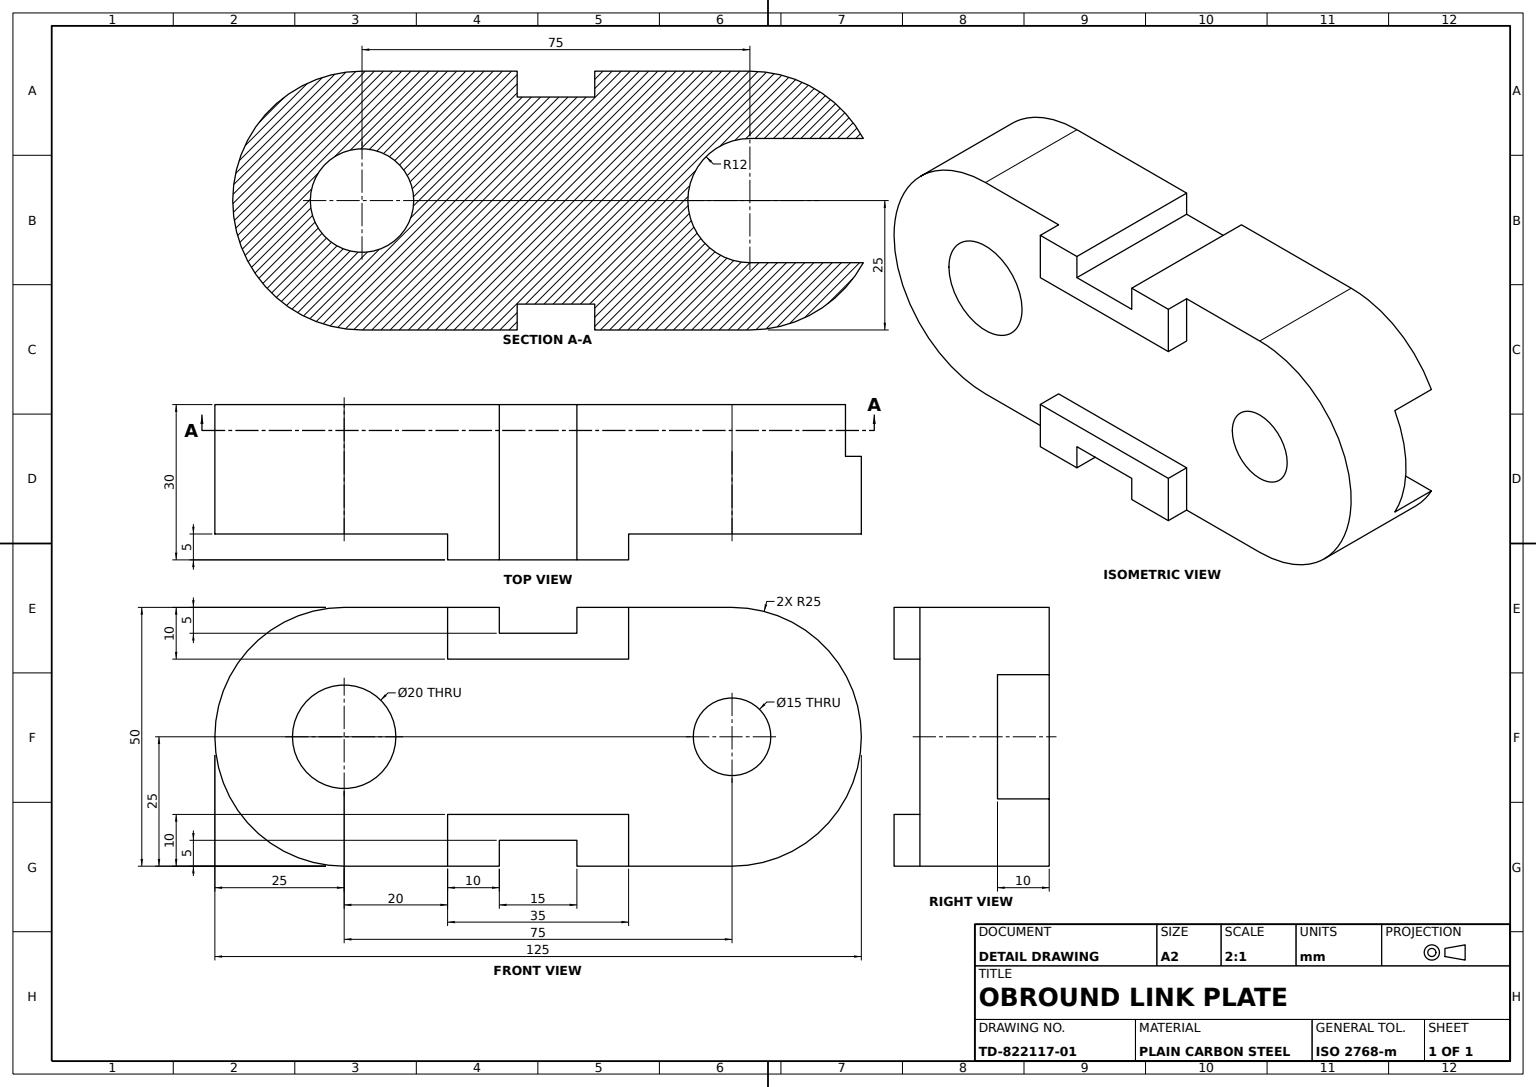
from build123d import *

# Parameters (mm, degrees)
LINK_BODY_DEPTH       = 25
SIDE_PADS_35X10_DEPTH = 5
T_SLOTS_DEPTH         = 35
CROSS_SLOT_12MM_DEPTH = 10
EYE_BORE_20_SKETCH_R  = 10
EYE_BORE_20_DEPTH     = 32
EYE_BORE_15_SKETCH_R  = 7.5
EYE_BORE_15_DEPTH     = 32


with BuildPart() as part:
    # Link Profile Sketch → Link Body (new body)
    with BuildSketch(Plane.XY):
        with BuildLine():
            Line((-37.5, 25), (37.5, 25))
            ThreePointArc((37.5, 25), (62.5, 0), (37.5, -25))
            Line((37.5, -25), (-37.5, -25))
            ThreePointArc((-37.5, -25), (-62.5, 0), (-37.5, 25))
        make_face()
    extrude(amount=LINK_BODY_DEPTH)

    # Side Pads Sketch → Side Pads 35x10 (add)
    with BuildSketch(Plane.XY.offset(25)):
        Polygon((0, -15), (17.5, -15), (17.5, -25), (-17.5, -25), (-17.5, -15), align=None)
        Polygon((-17.5, 15), (0, 15), (17.5, 15), (17.5, 25), (-17.5, 25), align=None)
    extrude(amount=SIDE_PADS_35X10_DEPTH)

    # T-Slots Sketch → T-Slots (cut)
    with BuildSketch(Plane.XY.offset(30)):
        Polygon((0, -20), (7.5, -20), (7.5, -26.538654193), (-7.5, -26.538654193), (-7.5, -20), align=None)
        Polygon((-7.5, 20), (0, 20), (7.5, 20), (7.5, 26.538654193), (-7.5, 26.538654193), align=None)
    extrude(amount=-T_SLOTS_DEPTH, mode=Mode.SUBTRACT)

    # Cross Slot Sketch → Cross Slot 12mm (cut)
    with BuildSketch(Plane(origin=(0, 0, 0), x_dir=(-1, 0, 0), z_dir=(0, 0, -1))):
        with BuildLine():
            Line((-37.5, 12), (-67.446025863, 12))
            Line((-67.446025863, 12), (-67.446025863, -12))
            Line((-67.446025863, -12), (-37.5, -12))
            ThreePointArc((-37.5, -12), (-25.5, 0), (-37.5, 12))
        make_face()
    extrude(amount=-CROSS_SLOT_12MM_DEPTH, mode=Mode.SUBTRACT)

    # Eye Bore Ø20 Sketch → Eye Bore Ø20 (cut)
    with BuildSketch(Plane.XY.offset(25)):
        with Locations((-37.5, 0)):
            Circle(EYE_BORE_20_SKETCH_R)
    extrude(amount=-EYE_BORE_20_DEPTH, mode=Mode.SUBTRACT)

    # Eye Bore Ø15 Sketch → Eye Bore Ø15 (cut)
    with BuildSketch(Plane.XY.offset(25)):
        with Locations((37.5, 0)):
            Circle(EYE_BORE_15_SKETCH_R)
    extrude(amount=-EYE_BORE_15_DEPTH, mode=Mode.SUBTRACT)


solid = part.part
